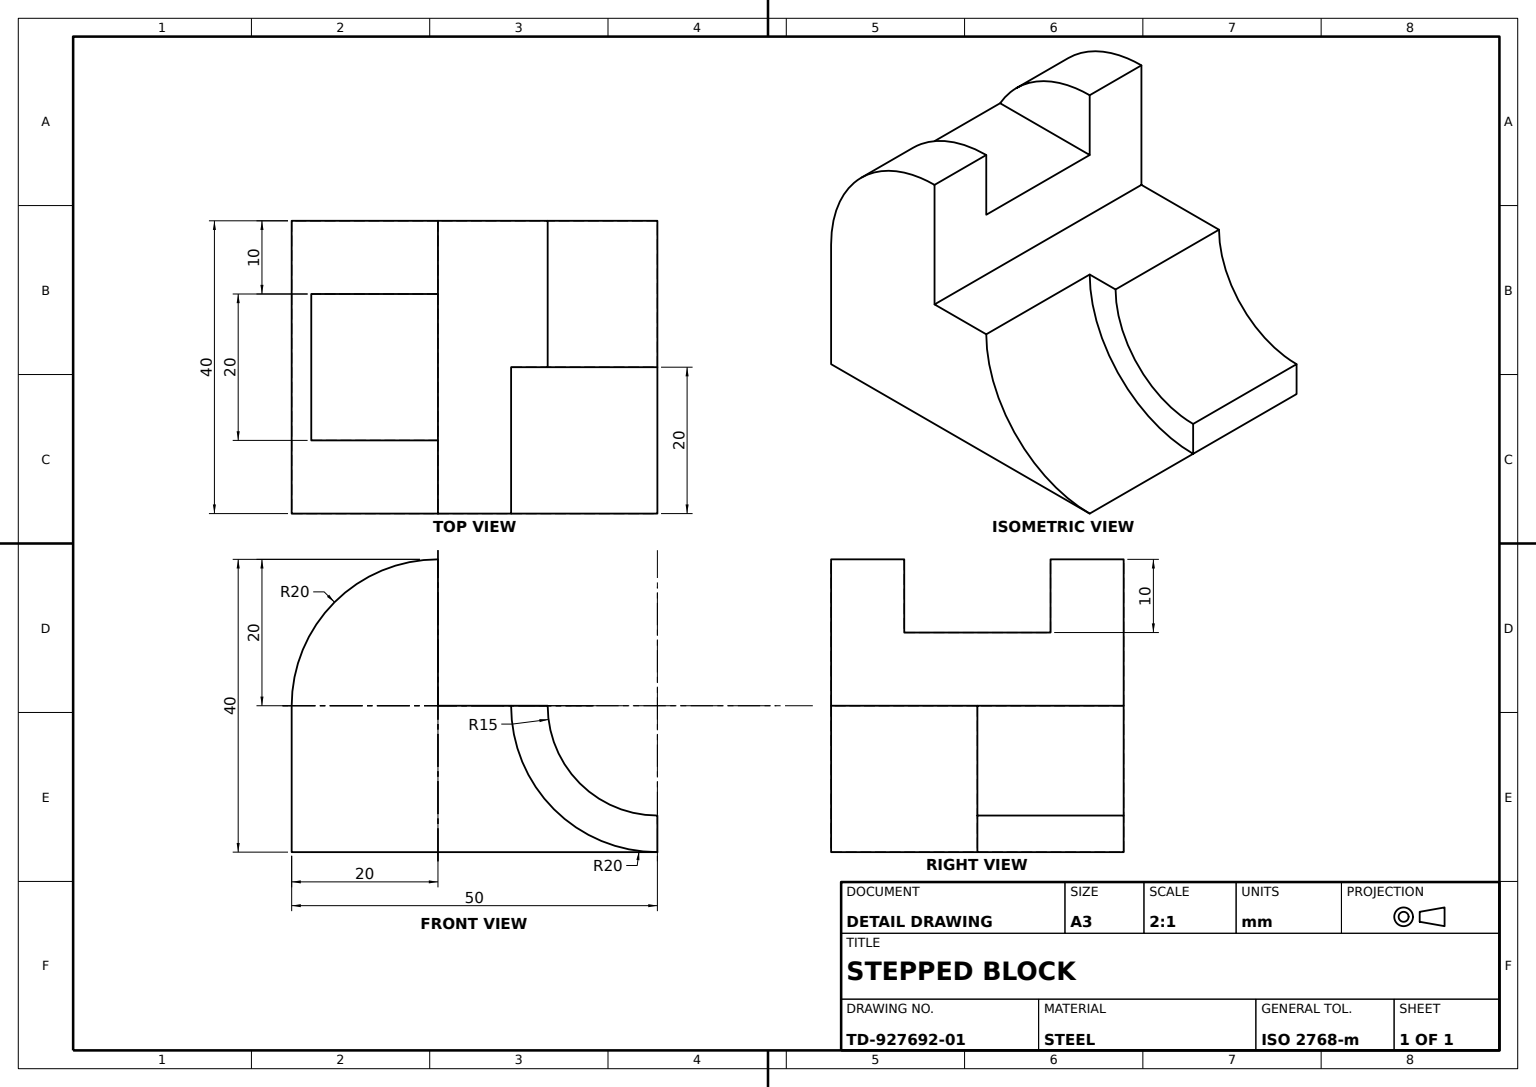
SolidWorks part; units mm, degrees
material "Plain Carbon Steel"
ref_plane "Front Plane" through (0, 0, 0) normal (0, 0, 1) x (1, 0, 0)
ref_plane "Top Plane" through (0, 0, 0) normal (0, 1, 0) x (1, 0, 0)
ref_plane "Right Plane" through (0, 0, 0) normal (1, 0, 0) x (0, 0, -1)
sketch "Base Block Profile" plane through (0, 0, 0) normal (0, 0, 1) x (1, 0, 0)
  line L1 (0, 0) -> (50, 0)
  line L2 (0, 0) -> (0, 40)
  line L3 (0, 40) -> (50, 40)
  line L4 (50, 0) -> (50, 40)
  dimension "D1" = 50
  dimension "D2" = 40
extrude "Base Block 50x40x40" add sketch "Base Block Profile" along normal mid plane 40
sketch "Corner Notch Profile" plane through (0, 0, 20) normal (0, 0, 1) x (1, 0, 0)
  line L1 (50, 40) -> (30, 40)
  line L2 (50, 40) -> (50, 20)
  line L3 (50, 20) -> (30, 20)
  line L4 (30, 40) -> (30, 20)
  dimension "D1" = 20
  dimension "D2" = 20
extrude "Corner Notch 20x20" cut sketch "Corner Notch Profile" against normal through all
sketch "Step Cut Profile" plane through (0, 0, 20) normal (0, 0, 1) x (1, 0, 0)
  line L0 (50, 0) -> (50, 20) construction
  line L1 (30, 20) -> (50, 20) construction
  line L2 (50, 0) -> (50, 20)
  line L3 (30, 20) -> (50, 20)
  arc A0 (30, 20) -> (50, 0) centre (50, 20) ccw
extrude "Step Cut" cut sketch "Step Cut Profile" against normal blind 20
sketch "Concave Arc Profile R30" plane through (0, 0, 0) normal (0, 0, 1) x (1, 0, 0)
  line L0 (50, 0) -> (50, 20) construction
  line L1 (50, 20) -> (30, 20) construction
  line L2 (50, 5) -> (50, 20)
  line L3 (50, 20) -> (35, 20)
  arc A0 (35, 20) -> (50, 5) centre (50, 20) ccw
  dimension "D1" = 30
extrude "Concave Arc Cut" cut sketch "Concave Arc Profile R30" against normal blind 20
sketch "Arc Groove Profile" plane through (0, 0, 20) normal (0, 0, 1) x (1, 0, 0)
  line L0 (0, 20) -> (35, 20) construction
  line L1 (0, 40) -> (0, 0) construction
  line L2 (20, 0) -> (20, 43.9713) construction
  line L5 (0, 40) -> (0, 20)
  line L6 (30, 40) -> (0, 40) construction
  line L7 (20, 40) -> (0, 40)
  arc A0 (35, 20) -> (50, 5) centre (50, 20) ccw construction
  arc A1 (20, 40) -> (0, 20) centre (20, 20) ccw
  dimension "D1" = 20
extrude "Arc Groove Cut" cut sketch "Arc Groove Profile" against normal through all
sketch "Top Slot Profile 10x10" plane through (0, 0, 0) normal (-1, 0, 0) x (0, 0, 1)
  line L2 (-10, 43.4082) -> (-10, 20)
  line L3 (-10, 20) -> (10, 20)
  line L4 (10, 43.4082) -> (10, 20)
  line L5 (-20, 20) -> (20, 20) construction
  line L6 (-10, 43.4082) -> (10, 43.4082)
  dimension "D1" = 10
  dimension "D2" = 10
  dimension "D3" = 23.4082
extrude "Top Slot 10x10" cut sketch "Top Slot Profile 10x10" against normal blind 20
sketch "Rounded Top Profile" plane through (0, 40, 0) normal (0, 1, 0) x (1, 0, 0)
  line L6 (20, 20) -> (20, 10)
  line L7 (20, 10) -> (20, -10)
  line L8 (20, -10) -> (20, -20)
  line L9 (20, -20) -> (30, -20)
  line L10 (30, -20) -> (30, 20)
  line L11 (30, 20) -> (20, 20)
  line L12 (20, 20) -> (20, 10)
  line L13 (20, 10) -> (20, -10)
  line L14 (20, -10) -> (20, -20)
  line L15 (20, -20) -> (30, -20)
  line L16 (30, -20) -> (30, 20)
  line L17 (30, 20) -> (20, 20)
  dimension "D1" = 0
extrude "Rounded Top Cut" cut sketch "Rounded Top Profile" against normal blind 20
sketch "Ridge Boss Profile" plane through (0, 20, 0) normal (0, 1, 0) x (1, 0, 0)
  line L0 (0, 10) -> (20, 10)
  line L1 (20, 10) -> (20, -10)
  line L2 (20, -10) -> (0, -10)
  line L3 (0, -10) -> (0, 10)
extrude "Ridge Boss 10" add sketch "Ridge Boss Profile" along normal blind 10
sketch "Ridge Round Profile" plane through (0, 0, 10) normal (0, 0, 1) x (1, 0, 0)
  line L2 (0, 30) -> (0, 20)
  line L3 (2.6795, 30) -> (0, 30)
  line L4 (0, 30) -> (0, 20)
  line L5 (2.6795, 30) -> (0, 30)
  arc A1 (2.6795, 30) -> (0, 20) centre (20, 20) ccw
  arc A2 (2.6795, 30) -> (0, 20) centre (20, 20) ccw
  dimension "D1" = 0
extrude "Ridge Round Cut" cut sketch "Ridge Round Profile" against normal blind 20
